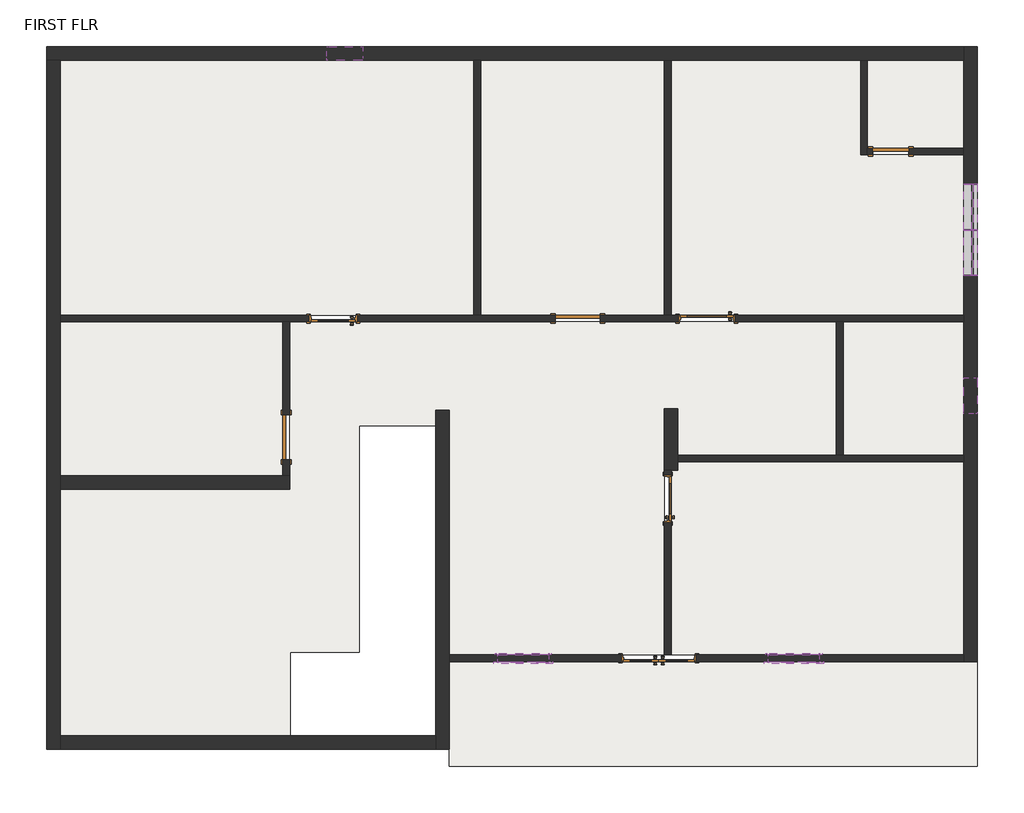
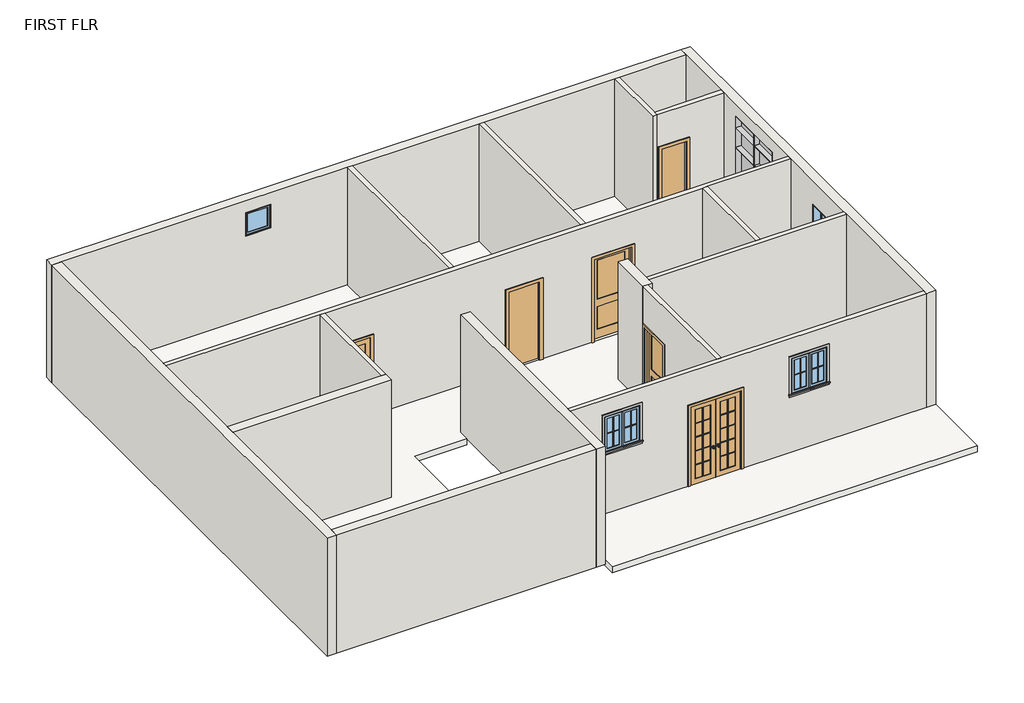
# One storey, incomplete: 22 members, 17 walls, 8 plates, 8 proxies, 7 doors, 4 windows, 2 slabs.
"""IFC4 building model written with IfcOpenShell, lengths in millimetres."""

from ifc_helpers import new_model, si_unit, frame, origin, place, context, project, spatial, polyline, outline, extrude, faceted_brep, transform, mapped, element, save
from components import muntin_pattern_2x2_muntin_pattern_2x2_b3fe6957, muntin_pattern_2x2_muntin_pattern_2x2_3e0ecaf2, trim_window_exterior_flat_with_sill_41619996, trim_window_interior_flat_picture_frame_51c85655, door_interior_double_full_glass_wood_double_door_glass_4_x_7_49a53587, door_d6fdea04, door_45c5d68b, door_049a69ed, door_d8f5dbb5, single_flush_bathroom_2_x_7_0bf9f8da, member_a87dc375, member_05d02c6e, member_049ff311, member_f4ca0770, member_d90fa784, member_091456ab, member_579a4f36, member_b53b5e8d, member_0fd823d9, member_acbd6ca0, system_panel_glazed_6813505b, system_panel_glazed_a35be92d, system_panel_glazed_bfd0fd53, system_panel_glazed_aaa2c267, window_80340324, window_a598f463

model = new_model("IFC4")

# Units and contexts
model_context = context("Model", 3, world=origin())
ifc_project = project(units=[si_unit("LENGTHUNIT", "METRE", prefix="MILLI")], contexts=[model_context])

# Site, building, storey
site = spatial("IfcSite", under=ifc_project)
building = spatial("IfcBuilding", under=site)
storey = spatial("IfcBuildingStorey", under=building, Name="FIRST FLR", Elevation=3352.8)

# Proxies
placement = place(None, origin())
muntin_pattern_2x2_muntin_pattern_2x2_shape = muntin_pattern_2x2_muntin_pattern_2x2_b3fe6957(model_context)
element("IfcBuildingElementProxy", 1, Name="Muntin Pattern_2x2 : Muntin Pattern_2x2", ObjectType="Muntin Pattern_2x2 : Muntin Pattern_2x2", at=placement, inside=storey, context=model_context, shape_type="MappedRepresentation", body=[
    mapped(muntin_pattern_2x2_muntin_pattern_2x2_shape, transform((2513.7983119, -4729.2803142, 5044.7639332), x_axis=(-1.0, 0.0, 0.0), y_axis=(0.0, -1.0, 0.0), z_axis=(0.0, 0.0, 1.0))),
])
element("IfcBuildingElementProxy", 2, Name="Muntin Pattern_2x2 : Muntin Pattern_2x2", ObjectType="Muntin Pattern_2x2 : Muntin Pattern_2x2", at=placement, inside=storey, context=model_context, shape_type="MappedRepresentation", body=[
    mapped(muntin_pattern_2x2_muntin_pattern_2x2_shape, transform((-2066.5321058, -4729.2803142, 5133.4876804), x_axis=(-1.0, 0.0, 0.0), y_axis=(0.0, -1.0, 0.0), z_axis=(0.0, 0.0, 1.0))),
])
muntin_pattern_2x2_muntin_pattern_2x2_2_shape = muntin_pattern_2x2_muntin_pattern_2x2_3e0ecaf2(model_context)
element("IfcBuildingElementProxy", 3, Name="Muntin Pattern_2x2 : Muntin Pattern_2x2", ObjectType="Muntin Pattern_2x2 : Muntin Pattern_2x2", at=placement, inside=storey, context=model_context, shape_type="MappedRepresentation", body=[
    mapped(muntin_pattern_2x2_muntin_pattern_2x2_2_shape, transform((2085.1733119, -4729.2803142, 5044.7639332), x_axis=(1.0, 0.0, 0.0), y_axis=(0.0, 1.0, 0.0), z_axis=(0.0, 0.0, 1.0))),
])
element("IfcBuildingElementProxy", 4, Name="Muntin Pattern_2x2 : Muntin Pattern_2x2", ObjectType="Muntin Pattern_2x2 : Muntin Pattern_2x2", at=placement, inside=storey, context=model_context, shape_type="MappedRepresentation", body=[
    mapped(muntin_pattern_2x2_muntin_pattern_2x2_2_shape, transform((-2495.1571058, -4729.2803142, 5133.4876804), x_axis=(1.0, 0.0, 0.0), y_axis=(0.0, 1.0, 0.0), z_axis=(0.0, 0.0, 1.0))),
])
trim_window_exterior_flat_with_sill_shape = trim_window_exterior_flat_with_sill_41619996(model_context)
element("IfcBuildingElementProxy", 5, Name="Trim-Window-Exterior-Flat : with Sill", ObjectType="Trim-Window-Exterior-Flat : with Sill", at=placement, inside=storey, context=model_context, shape_type="MappedRepresentation", body=[
    mapped(trim_window_exterior_flat_with_sill_shape, transform((2299.4858119, -4738.8053142, 5889.3139332), x_axis=(1.0, 0.0, 0.0), y_axis=(0.0, 0.0, 1.0), z_axis=(0.0, -1.0, 0.0))),
])
element("IfcBuildingElementProxy", 6, Name="Trim-Window-Exterior-Flat : with Sill", ObjectType="Trim-Window-Exterior-Flat : with Sill", at=placement, inside=storey, context=model_context, shape_type="MappedRepresentation", body=[
    mapped(trim_window_exterior_flat_with_sill_shape, transform((-2280.8446058, -4738.8053142, 5978.0376804), x_axis=(1.0, 0.0, 0.0), y_axis=(0.0, 0.0, 1.0), z_axis=(0.0, -1.0, 0.0))),
])
trim_window_interior_flat_picture_frame_shape = trim_window_interior_flat_picture_frame_51c85655(model_context)
element("IfcBuildingElementProxy", 7, Name="Trim-Window-Interior-Flat : Picture Frame", ObjectType="Trim-Window-Interior-Flat : Picture Frame", at=placement, inside=storey, context=model_context, shape_type="MappedRepresentation", body=[
    mapped(trim_window_interior_flat_picture_frame_shape, transform((2299.4858119, -4624.5053142, 5889.3139332), x_axis=(-1.0, 0.0, 0.0), y_axis=(0.0, 0.0, 1.0), z_axis=(0.0, 1.0, 0.0))),
])
element("IfcBuildingElementProxy", 8, Name="Trim-Window-Interior-Flat : Picture Frame", ObjectType="Trim-Window-Interior-Flat : Picture Frame", at=placement, inside=storey, context=model_context, shape_type="MappedRepresentation", body=[
    mapped(trim_window_interior_flat_picture_frame_shape, transform((-2280.8446058, -4624.5053142, 5978.0376804), x_axis=(-1.0, 0.0, 0.0), y_axis=(0.0, 0.0, 1.0), z_axis=(0.0, 1.0, 0.0))),
])

# Doors
door_interior_double_full_glass_wood_double_door_glass_4_x_7_shape = door_interior_double_full_glass_wood_double_door_glass_4_x_7_49a53587(model_context)
element("IfcDoor", 9, ObjectType="Door-Interior-Double-Full Glass-Wood : DOUBLE DOOR GLASS 4' X 7'", at=placement, inside=storey, context=model_context, shape_type="MappedRepresentation", body=[
    mapped(door_interior_double_full_glass_wood_double_door_glass_4_x_7_shape, transform((13.4858119, -4684.8303142, 3352.8), x_axis=(-1.0, 0.0, 0.0), y_axis=(0.0, -1.0, 0.0), z_axis=(0.0, 0.0, 1.0))),
])
door_shape = door_d6fdea04(model_context)
element("IfcDoor", 10, ObjectType="Door-Interior-Single-2_Panel-Wood : 30\" x 80\"", at=placement, inside=storey, context=model_context, shape_type="MappedRepresentation", body=[
    mapped(door_shape, transform((169.0608119, -1978.5424275, 3352.8), x_axis=(0.0, 1.0, 0.0), y_axis=(-1.0, 0.0, 0.0), z_axis=(0.0, 0.0, 1.0))),
])
door_2_shape = door_45c5d68b(model_context)
element("IfcDoor", 11, ObjectType="Door-Interior-Single-2_Panel-Wood : 30\" x 80\"", at=placement, inside=storey, context=model_context, shape_type="MappedRepresentation", body=[
    mapped(door_2_shape, transform((-5499.9044923, 1067.2421668, 3352.8), x_axis=(-1.0, 0.0, 0.0), y_axis=(0.0, -1.0, 0.0), z_axis=(0.0, 0.0, 1.0))),
])
door_3_shape = door_049a69ed(model_context)
element("IfcDoor", 12, ObjectType="Door-Interior-Single-2_Panel-Wood : 36\" x 84\"", at=placement, inside=storey, context=model_context, shape_type="MappedRepresentation", body=[
    mapped(door_3_shape, transform((824.7020146, 1073.5921668, 3352.8), x_axis=(-1.0, 0.0, 0.0), y_axis=(0.0, -1.0, 0.0), z_axis=(0.0, 0.0, 1.0))),
])
door_4_shape = door_d8f5dbb5(model_context)
element("IfcDoor", 13, ObjectType="Single-Flush : 30\" x 80\"", at=placement, inside=storey, context=model_context, shape_type="MappedRepresentation", body=[
    mapped(door_4_shape, transform((-1359.6979854, 1070.4171668, 3352.8), x_axis=(1.0, 0.0, 0.0), y_axis=(0.0, 1.0, 0.0), z_axis=(0.0, 0.0, 1.0))),
])
element("IfcDoor", 14, ObjectType="Single-Flush : 30\" x 80\"", at=placement, inside=storey, context=model_context, shape_type="MappedRepresentation", body=[
    mapped(door_4_shape, transform((-6295.715751, -942.6707851, 3352.8), x_axis=(0.0, 1.0, 0.0), y_axis=(-1.0, 0.0, 0.0), z_axis=(0.0, 0.0, 1.0))),
])
single_flush_bathroom_2_x_7_shape = single_flush_bathroom_2_x_7_0bf9f8da(model_context)
element("IfcDoor", 15, ObjectType="Single-Flush : BATHROOM 2' X 7'", at=placement, inside=storey, context=model_context, shape_type="MappedRepresentation", body=[
    mapped(single_flush_bathroom_2_x_7_shape, transform((3941.8301763, 3897.1946858, 3352.8), x_axis=(-1.0, 0.0, 0.0), y_axis=(0.0, -1.0, 0.0), z_axis=(0.0, 0.0, 1.0))),
])

# Members
member_shape = member_a87dc375(model_context)
element("IfcMember", 16, ObjectType="Rectangular Mullion : 2.5\" x 5\" rectangular", at=placement, inside=storey, context=model_context, shape_type="MappedRepresentation", body=[
    mapped(member_shape, transform((5293.034249, 2571.0346634, 3352.8), x_axis=(0.0, -1.0, 0.0), y_axis=(-1.0, 0.0, 0.0), z_axis=(0.0, 0.0, -1.0))),
])
member_2_shape = member_05d02c6e(model_context)
element("IfcMember", 17, ObjectType="Rectangular Mullion : 2.5\" x 5\" rectangular", at=placement, inside=storey, context=model_context, shape_type="MappedRepresentation", body=[
    mapped(member_2_shape, transform((5293.034249, 2571.0346634, 4216.4), x_axis=(0.0, -1.0, 0.0), y_axis=(-1.0, 0.0, 0.0), z_axis=(0.0, 0.0, -1.0))),
])
member_3_shape = member_049ff311(model_context)
element("IfcMember", 18, ObjectType="Rectangular Mullion : 2.5\" x 5\" rectangular", at=placement, inside=storey, context=model_context, shape_type="MappedRepresentation", body=[
    mapped(member_3_shape, transform((5293.034249, 1793.1596634, 3352.8), x_axis=(0.0, -1.0, 0.0), y_axis=(-1.0, 0.0, 0.0), z_axis=(0.0, 0.0, -1.0))),
])
member_4_shape = member_f4ca0770(model_context)
element("IfcMember", 19, ObjectType="Rectangular Mullion : 2.5\" x 5\" rectangular", at=placement, inside=storey, context=model_context, shape_type="MappedRepresentation", body=[
    mapped(member_4_shape, transform((5293.034249, 3348.9096634, 5283.2), x_axis=(0.0, 1.0, 0.0), y_axis=(-1.0, 0.0, 0.0), z_axis=(0.0, 0.0, 1.0))),
])
element("IfcMember", 20, ObjectType="Rectangular Mullion : 2.5\" x 5\" rectangular", at=placement, inside=storey, context=model_context, shape_type="MappedRepresentation", body=[
    mapped(member_4_shape, transform((5293.034249, 1793.1596634, 4216.4), x_axis=(0.0, -1.0, 0.0), y_axis=(-1.0, 0.0, 0.0), z_axis=(0.0, 0.0, -1.0))),
])
element("IfcMember", 21, ObjectType="Rectangular Mullion : 2.5\" x 5\" rectangular", at=placement, inside=storey, context=model_context, shape_type="MappedRepresentation", body=[
    mapped(member_3_shape, transform((5293.034249, 3348.9096634, 4216.4), x_axis=(0.0, 1.0, 0.0), y_axis=(-1.0, 0.0, 0.0), z_axis=(0.0, 0.0, 1.0))),
])
member_5_shape = member_d90fa784(model_context)
element("IfcMember", 22, ObjectType="Rectangular Mullion : 2.5\" x 5\" rectangular", at=placement, inside=storey, context=model_context, shape_type="MappedRepresentation", body=[
    mapped(member_5_shape, transform((5293.034249, 1800.3986634, 6096.0), x_axis=(0.0, 0.0, 1.0), y_axis=(-1.0, 0.0, 0.0), z_axis=(0.0, -1.0, 0.0))),
])
element("IfcMember", 23, ObjectType="Rectangular Mullion : 2.5\" x 5\" rectangular", at=placement, inside=storey, context=model_context, shape_type="MappedRepresentation", body=[
    mapped(member_5_shape, transform((5293.034249, 2574.6541634, 6096.0), x_axis=(0.0, 0.0, 1.0), y_axis=(-1.0, 0.0, 0.0), z_axis=(0.0, -1.0, 0.0))),
])
element("IfcMember", 24, ObjectType="Rectangular Mullion : 2.5\" x 5\" rectangular", at=placement, inside=storey, context=model_context, shape_type="MappedRepresentation", body=[
    mapped(member_5_shape, transform((5293.034249, 3341.6706634, 3352.8), x_axis=(0.0, 0.0, -1.0), y_axis=(-1.0, 0.0, 0.0), z_axis=(0.0, 1.0, 0.0))),
])
element("IfcMember", 25, ObjectType="Rectangular Mullion : 2.5\" x 5\" rectangular", at=placement, inside=storey, context=model_context, shape_type="MappedRepresentation", body=[
    mapped(member_5_shape, transform((5293.034249, 2567.4151634, 3352.8), x_axis=(0.0, 0.0, -1.0), y_axis=(-1.0, 0.0, 0.0), z_axis=(0.0, 1.0, 0.0))),
])
member_6_shape = member_091456ab(model_context)
element("IfcMember", 26, ObjectType="Rectangular Mullion : 2.5\" x 5\" rectangular", at=placement, inside=storey, context=model_context, shape_type="MappedRepresentation", body=[
    mapped(member_6_shape, transform((5293.034249, 2574.6541634, 5283.2), x_axis=(0.0, 0.0, 1.0), y_axis=(-1.0, 0.0, 0.0), z_axis=(0.0, -1.0, 0.0))),
])
element("IfcMember", 27, ObjectType="Rectangular Mullion : 2.5\" x 5\" rectangular", at=placement, inside=storey, context=model_context, shape_type="MappedRepresentation", body=[
    mapped(member_6_shape, transform((5293.034249, 1800.3986634, 5283.2), x_axis=(0.0, 0.0, 1.0), y_axis=(-1.0, 0.0, 0.0), z_axis=(0.0, -1.0, 0.0))),
])
element("IfcMember", 28, ObjectType="Rectangular Mullion : 2.5\" x 5\" rectangular", at=placement, inside=storey, context=model_context, shape_type="MappedRepresentation", body=[
    mapped(member_6_shape, transform((5293.034249, 2574.6541634, 4216.4), x_axis=(0.0, 0.0, 1.0), y_axis=(-1.0, 0.0, 0.0), z_axis=(0.0, -1.0, 0.0))),
])
element("IfcMember", 29, ObjectType="Rectangular Mullion : 2.5\" x 5\" rectangular", at=placement, inside=storey, context=model_context, shape_type="MappedRepresentation", body=[
    mapped(member_6_shape, transform((5293.034249, 1800.3986634, 4216.4), x_axis=(0.0, 0.0, 1.0), y_axis=(-1.0, 0.0, 0.0), z_axis=(0.0, -1.0, 0.0))),
])
element("IfcMember", 30, ObjectType="Rectangular Mullion : 2.5\" x 5\" rectangular", at=placement, inside=storey, context=model_context, shape_type="MappedRepresentation", body=[
    mapped(member_6_shape, transform((5293.034249, 2574.6541634, 5791.2), x_axis=(0.0, 0.0, 1.0), y_axis=(-1.0, 0.0, 0.0), z_axis=(0.0, -1.0, 0.0))),
])
element("IfcMember", 31, ObjectType="Rectangular Mullion : 2.5\" x 5\" rectangular", at=placement, inside=storey, context=model_context, shape_type="MappedRepresentation", body=[
    mapped(member_6_shape, transform((5293.034249, 1800.3986634, 5791.2), x_axis=(0.0, 0.0, 1.0), y_axis=(-1.0, 0.0, 0.0), z_axis=(0.0, -1.0, 0.0))),
])
member_7_shape = member_579a4f36(model_context)
element("IfcMember", 32, ObjectType="Rectangular Mullion : 2.5\" x 5\" rectangular", at=placement, inside=storey, context=model_context, shape_type="MappedRepresentation", body=[
    mapped(member_7_shape, transform((5293.034249, 1793.1596634, 5791.2), x_axis=(0.0, -1.0, 0.0), y_axis=(-1.0, 0.0, 0.0), z_axis=(0.0, 0.0, -1.0))),
])
element("IfcMember", 33, ObjectType="Rectangular Mullion : 2.5\" x 5\" rectangular", at=placement, inside=storey, context=model_context, shape_type="MappedRepresentation", body=[
    mapped(member_7_shape, transform((5293.034249, 3348.9096634, 6096.0), x_axis=(0.0, 1.0, 0.0), y_axis=(-1.0, 0.0, 0.0), z_axis=(0.0, 0.0, 1.0))),
])
member_8_shape = member_b53b5e8d(model_context)
element("IfcMember", 34, ObjectType="Rectangular Mullion : 2.5\" x 5\" rectangular", at=placement, inside=storey, context=model_context, shape_type="MappedRepresentation", body=[
    mapped(member_8_shape, transform((5293.034249, 2571.0346634, 5791.2), x_axis=(0.0, -1.0, 0.0), y_axis=(-1.0, 0.0, 0.0), z_axis=(0.0, 0.0, -1.0))),
])
member_9_shape = member_0fd823d9(model_context)
element("IfcMember", 35, ObjectType="Rectangular Mullion : 2.5\" x 5\" rectangular", at=placement, inside=storey, context=model_context, shape_type="MappedRepresentation", body=[
    mapped(member_9_shape, transform((5293.034249, 2571.0346634, 5283.2), x_axis=(0.0, -1.0, 0.0), y_axis=(-1.0, 0.0, 0.0), z_axis=(0.0, 0.0, -1.0))),
])
member_10_shape = member_acbd6ca0(model_context)
element("IfcMember", 36, ObjectType="Rectangular Mullion : 2.5\" x 5\" rectangular", at=placement, inside=storey, context=model_context, shape_type="MappedRepresentation", body=[
    mapped(member_10_shape, transform((5293.034249, 1793.1596634, 5283.2), x_axis=(0.0, -1.0, 0.0), y_axis=(-1.0, 0.0, 0.0), z_axis=(0.0, 0.0, -1.0))),
])
element("IfcMember", 37, ObjectType="Rectangular Mullion : 2.5\" x 5\" rectangular", at=placement, inside=storey, context=model_context, shape_type="MappedRepresentation", body=[
    mapped(member_10_shape, transform((5293.034249, 3348.9096634, 5791.2), x_axis=(0.0, 1.0, 0.0), y_axis=(-1.0, 0.0, 0.0), z_axis=(0.0, 0.0, 1.0))),
])

# Plates
system_panel_glazed_shape = system_panel_glazed_6813505b(model_context)
element("IfcPlate", 38, ObjectType="System Panel : Glazed", at=placement, inside=storey, context=model_context, shape_type="MappedRepresentation", body=[
    mapped(system_panel_glazed_shape, transform((5293.034249, 2958.1624134, 3360.039), x_axis=(0.0, -1.0, 0.0), y_axis=(1.0, 0.0, 0.0), z_axis=(0.0, 0.0, 1.0))),
])
element("IfcPlate", 39, ObjectType="System Panel : Glazed", at=placement, inside=storey, context=model_context, shape_type="MappedRepresentation", body=[
    mapped(system_panel_glazed_shape, transform((5293.034249, 2183.9069134, 3360.039), x_axis=(0.0, -1.0, 0.0), y_axis=(1.0, 0.0, 0.0), z_axis=(0.0, 0.0, 1.0))),
])
system_panel_glazed_2_shape = system_panel_glazed_a35be92d(model_context)
element("IfcPlate", 40, ObjectType="System Panel : Glazed", at=placement, inside=storey, context=model_context, shape_type="MappedRepresentation", body=[
    mapped(system_panel_glazed_2_shape, transform((5293.034249, 2958.1624134, 4220.0195), x_axis=(0.0, -1.0, 0.0), y_axis=(1.0, 0.0, 0.0), z_axis=(0.0, 0.0, 1.0))),
])
element("IfcPlate", 41, ObjectType="System Panel : Glazed", at=placement, inside=storey, context=model_context, shape_type="MappedRepresentation", body=[
    mapped(system_panel_glazed_2_shape, transform((5293.034249, 2183.9069134, 4220.0195), x_axis=(0.0, -1.0, 0.0), y_axis=(1.0, 0.0, 0.0), z_axis=(0.0, 0.0, 1.0))),
])
system_panel_glazed_3_shape = system_panel_glazed_bfd0fd53(model_context)
element("IfcPlate", 42, ObjectType="System Panel : Glazed", at=placement, inside=storey, context=model_context, shape_type="MappedRepresentation", body=[
    mapped(system_panel_glazed_3_shape, transform((5293.034249, 2958.1624134, 5286.8195), x_axis=(0.0, -1.0, 0.0), y_axis=(1.0, 0.0, 0.0), z_axis=(0.0, 0.0, 1.0))),
])
element("IfcPlate", 43, ObjectType="System Panel : Glazed", at=placement, inside=storey, context=model_context, shape_type="MappedRepresentation", body=[
    mapped(system_panel_glazed_3_shape, transform((5293.034249, 2183.9069134, 5286.8195), x_axis=(0.0, -1.0, 0.0), y_axis=(1.0, 0.0, 0.0), z_axis=(0.0, 0.0, 1.0))),
])
system_panel_glazed_4_shape = system_panel_glazed_aaa2c267(model_context)
element("IfcPlate", 44, ObjectType="System Panel : Glazed", at=placement, inside=storey, context=model_context, shape_type="MappedRepresentation", body=[
    mapped(system_panel_glazed_4_shape, transform((5293.034249, 2958.1624134, 5794.8195), x_axis=(0.0, -1.0, 0.0), y_axis=(1.0, 0.0, 0.0), z_axis=(0.0, 0.0, 1.0))),
])
element("IfcPlate", 45, ObjectType="System Panel : Glazed", at=placement, inside=storey, context=model_context, shape_type="MappedRepresentation", body=[
    mapped(system_panel_glazed_4_shape, transform((5293.034249, 2183.9069134, 5794.8195), x_axis=(0.0, -1.0, 0.0), y_axis=(1.0, 0.0, 0.0), z_axis=(0.0, 0.0, 1.0))),
])

# Slabs
element("IfcSlab", 46, ObjectType="MARBLE FLOORING 6\"", at=placement, inside=storey, context=model_context, shape_type="SweptSolid", body=[
    extrude(outline(polyline([(-3118.6544923, 5446.5946858), (-3118.6544923, 1127.5671668), (-10124.765751, 1127.5671668), (-10124.765751, 5446.5946858), (-3118.6544923, 5446.5946858)])), frame((0.0, 0.0, 3200.4), z_axis=(0.0, 0.0, 1.0), x_axis=(1.0, 0.0, 0.0)), (0.0, 0.0, 1.0), 152.4),
    extrude(outline(polyline([(107.1520146, 5446.5946858), (107.1520146, 1127.5671668), (-3004.3544923, 1127.5671668), (-3004.3544923, 5446.5946858), (107.1520146, 5446.5946858)])), frame((0.0, 0.0, 3200.4), z_axis=(0.0, 0.0, 1.0), x_axis=(1.0, 0.0, 0.0)), (0.0, 0.0, 1.0), 152.4),
    extrude(outline(polyline([(3427.4801763, 5446.5946858), (3427.4801763, 3840.0446858), (5178.734249, 3840.0446858), (5178.734249, 1127.5671668), (221.4520146, 1127.5671668), (221.4520146, 5446.5946858), (3427.4801763, 5446.5946858)])), frame((0.0, 0.0, 3200.4), z_axis=(0.0, 0.0, 1.0), x_axis=(1.0, 0.0, 0.0)), (0.0, 0.0, 1.0), 152.4),
    extrude(outline(polyline([(5178.734249, 5446.5946858), (5178.734249, 3954.3446858), (3541.7801763, 3954.3446858), (3541.7801763, 5446.5946858), (5178.734249, 5446.5946858)])), frame((0.0, 0.0, 3200.4), z_axis=(0.0, 0.0, 1.0), x_axis=(1.0, 0.0, 0.0)), (0.0, 0.0, 1.0), 152.4),
    extrude(outline(polyline([(5178.734249, 1013.2671668), (5178.734249, -1243.1716798), (3134.034249, -1243.1716798), (3134.034249, 1013.2671668), (5178.734249, 1013.2671668)])), frame((0.0, 0.0, 3200.4), z_axis=(0.0, 0.0, 1.0), x_axis=(1.0, 0.0, 0.0)), (0.0, 0.0, 1.0), 152.4),
    extrude(outline(polyline([(-6352.865751, 1013.2671668), (-6352.865751, -1590.3707851), (-10124.765751, -1590.3707851), (-10124.765751, 1013.2671668), (-6352.865751, 1013.2671668)])), frame((0.0, 0.0, 3200.4), z_axis=(0.0, 0.0, 1.0), x_axis=(1.0, 0.0, 0.0)), (0.0, 0.0, 1.0), 152.4),
    extrude(outline(polyline([(223.0358119, -4624.5053142), (223.0358119, -1495.9424275), (337.3358119, -1495.9424275), (337.3358119, -1357.4716798), (5178.734249, -1357.4716798), (5178.734249, -4624.5053142), (223.0358119, -4624.5053142)])), frame((0.0, 0.0, 3200.4), z_axis=(0.0, 0.0, 1.0), x_axis=(1.0, 0.0, 0.0)), (0.0, 0.0, 1.0), 152.4),
    extrude(outline(polyline([(-10124.765751, -1818.9707851), (-6238.565751, -1818.9707851), (-6238.565751, 1013.2671668), (3019.734249, 1013.2671668), (3019.734249, -1243.1716798), (337.3358119, -1243.1716798), (337.3358119, -454.5424275), (108.7358119, -454.5424275), (108.7358119, -4624.5053142), (-3538.1446058, -4624.5053142), (-3538.1446058, -484.3053142), (-3766.7446058, -484.3053142), (-3766.7446058, -746.7863315), (-5057.7237749, -746.7863315), (-5057.7237749, -4582.1863315), (-6226.1237749, -4582.1863315), (-6226.1237749, -5996.1053142), (-10124.765751, -5996.1053142), (-10124.765751, -1818.9707851)])), frame((0.0, 0.0, 3200.4), z_axis=(0.0, 0.0, 1.0), x_axis=(1.0, 0.0, 0.0)), (0.0, 0.0, 1.0), 152.4),
])
element("IfcSlab", 47, ObjectType="MARBLE FLOORING 6\"", at=placement, inside=storey, context=model_context, shape_type="SweptSolid", body=[
    extrude(outline(polyline([(5407.334249, -4738.8053142), (5407.334249, -6508.7205873), (-3538.1446058, -6508.7205873), (-3538.1446058, -4738.8053142), (5407.334249, -4738.8053142)])), frame((0.0, 0.0, 3302.0), z_axis=(0.0, 0.0, 1.0), x_axis=(1.0, 0.0, 0.0)), (0.0, 0.0, 1.0), 152.4),
])

# Walls
element("IfcWall", 48, at=placement, inside=storey, context=model_context, shape_type="SweptSolid", body=[
    extrude(outline(polyline([(-3766.7446058, -6224.7053142), (-10124.765751, -6224.7053142), (-10124.765751, -5996.1053142), (-3766.7446058, -5996.1053142), (-3766.7446058, -6224.7053142)])), frame((0.0, 0.0, 3352.8), z_axis=(0.0, 0.0, 1.0), x_axis=(1.0, 0.0, 0.0)), (0.0, 0.0, 1.0), 3048.0),
])
element("IfcWall", 49, at=placement, inside=storey, context=model_context, shape_type="Brep", body=[
    faceted_brep([(5407.334249, 5675.1946858, 6400.8), (5407.334249, -4738.8053142, 6400.8), (5407.334249, -4738.8053142, 3352.8), (5407.334249, 1793.1596634, 3352.8), (5407.334249, 1793.1596634, 6096.0), (5407.334249, 3348.9096634, 6096.0), (5407.334249, 3348.9096634, 3352.8), (5407.334249, 5675.1946858, 3352.8), (5407.334249, -538.3216798, 5791.2), (5407.334249, 71.2783202, 5791.2), (5407.334249, 71.2783202, 5181.6), (5407.334249, -538.3216798, 5181.6), (5178.734249, -4738.8053142, 6400.8), (5178.734249, -4624.5053142, 6400.8), (5178.734249, -1357.4716798, 6400.8), (5178.734249, -1243.1716798, 6400.8), (5178.734249, 1013.2671668, 6400.8), (5178.734249, 1127.5671668, 6400.8), (5178.734249, 3840.0446858, 6400.8), (5178.734249, 3954.3446858, 6400.8), (5178.734249, 5446.5946858, 6400.8), (5178.734249, 5675.1946858, 6400.8), (5178.734249, 5675.1946858, 3352.8), (5178.734249, 5446.5946858, 3352.8), (5178.734249, 3954.3446858, 3352.8), (5178.734249, 3840.0446858, 3352.8), (5178.734249, 3348.9096634, 3352.8), (5178.734249, 3348.9096634, 6096.0), (5178.734249, 1793.1596634, 6096.0), (5178.734249, 1793.1596634, 3352.8), (5178.734249, 1127.5671668, 3352.8), (5178.734249, 1013.2671668, 3352.8), (5178.734249, -1243.1716798, 3352.8), (5178.734249, -1357.4716798, 3352.8), (5178.734249, -4624.5053142, 3352.8), (5178.734249, -4738.8053142, 3352.8), (5178.734249, -538.3216798, 5791.2), (5178.734249, -538.3216798, 5181.6), (5178.734249, 71.2783202, 5181.6), (5178.734249, 71.2783202, 5791.2)], [[[0, 1, 2, 3, 4, 5, 6, 7], [8, 9, 10, 11]], [[12, 13, 14, 15, 16, 17, 18, 19, 20, 21, 22, 23, 24, 25, 26, 27, 28, 29, 30, 31, 32, 33, 34, 35], [36, 37, 38, 39]], [[2, 35, 34, 33, 32, 31, 30, 29, 3]], [[22, 7, 6, 26, 25, 24, 23]], [[1, 0, 21, 20, 19, 18, 17, 16, 15, 14, 13, 12]], [[2, 1, 12, 35]], [[0, 7, 22, 21]], [[5, 27, 26, 6]], [[27, 5, 4, 28]], [[28, 4, 3, 29]], [[37, 36, 8, 11]], [[38, 37, 11, 10]], [[39, 38, 10, 9]], [[36, 39, 9, 8]]]),
])
element("IfcWall", 50, at=placement, inside=storey, context=model_context, shape_type="Brep", body=[
    faceted_brep([(5178.734249, 5675.1946858, 3352.8), (-10353.365751, 5675.1946858, 3352.8), (-10353.365751, 5675.1946858, 6400.8), (5178.734249, 5675.1946858, 6400.8), (-5608.7434923, 5675.1946858, 6096.0), (-5608.7434923, 5675.1946858, 5486.4), (-4999.1434923, 5675.1946858, 5486.4), (-4999.1434923, 5675.1946858, 6096.0), (5178.734249, 5446.5946858, 3352.8), (5178.734249, 5446.5946858, 6400.8), (3541.7801763, 5446.5946858, 6400.8), (3427.4801763, 5446.5946858, 6400.8), (221.4520146, 5446.5946858, 6400.8), (107.1520146, 5446.5946858, 6400.8), (-3004.3544923, 5446.5946858, 6400.8), (-3118.6544923, 5446.5946858, 6400.8), (-10124.765751, 5446.5946858, 6400.8), (-10353.365751, 5446.5946858, 6400.8), (-10353.365751, 5446.5946858, 3352.8), (-10124.765751, 5446.5946858, 3352.8), (-3118.6544923, 5446.5946858, 3352.8), (-3004.3544923, 5446.5946858, 3352.8), (107.1520146, 5446.5946858, 3352.8), (221.4520146, 5446.5946858, 3352.8), (3427.4801763, 5446.5946858, 3352.8), (3541.7801763, 5446.5946858, 3352.8), (-5608.7434923, 5446.5946858, 6096.0), (-4999.1434923, 5446.5946858, 6096.0), (-4999.1434923, 5446.5946858, 5486.4), (-5608.7434923, 5446.5946858, 5486.4)], [[[0, 1, 2, 3], [4, 5, 6, 7]], [[8, 9, 10, 11, 12, 13, 14, 15, 16, 17, 18, 19, 20, 21, 22, 23, 24, 25], [26, 27, 28, 29]], [[1, 0, 8, 25, 24, 23, 22, 21, 20, 19, 18]], [[3, 2, 17, 16, 15, 14, 13, 12, 11, 10, 9]], [[0, 3, 9, 8]], [[2, 1, 18, 17]], [[5, 4, 26, 29]], [[6, 5, 29, 28]], [[7, 6, 28, 27]], [[4, 7, 27, 26]]]),
])
element("IfcWall", 51, at=placement, inside=storey, context=model_context, shape_type="Brep", body=[
    faceted_brep([(-10353.365751, 5446.5946858, 3352.8), (-10353.365751, -6224.7053142, 3352.8), (-10353.365751, -6224.7053142, 6400.8), (-10353.365751, 5446.5946858, 6400.8), (-10124.765751, 5446.5946858, 3352.8), (-10124.765751, 5446.5946858, 6400.8), (-10124.765751, 1127.5671668, 6400.8), (-10124.765751, 1013.2671668, 6400.8), (-10124.765751, -1590.3707851, 6400.8), (-10124.765751, -1818.9707851, 6400.8), (-10124.765751, -5996.1053142, 6400.8), (-10124.765751, -6224.7053142, 6400.8), (-10124.765751, -6224.7053142, 3352.8), (-10124.765751, -5996.1053142, 3352.8), (-10124.765751, -1818.9707851, 3352.8), (-10124.765751, -1590.3707851, 3352.8), (-10124.765751, 1013.2671668, 3352.8), (-10124.765751, 1127.5671668, 3352.8)], [[[0, 1, 2, 3]], [[4, 5, 6, 7, 8, 9, 10, 11, 12, 13, 14, 15, 16, 17]], [[1, 0, 4, 17, 16, 15, 14, 13, 12]], [[3, 2, 11, 10, 9, 8, 7, 6, 5]], [[0, 3, 5, 4]], [[2, 1, 12, 11]]]),
])
element("IfcWall", 52, at=placement, inside=storey, context=model_context, shape_type="Brep", body=[
    faceted_brep([(-10124.765751, -1818.9707851, 3352.8), (-6238.565751, -1818.9707851, 3352.8), (-6238.565751, -1818.9707851, 6400.8), (-10124.765751, -1818.9707851, 6400.8), (-10124.765751, -1590.3707851, 3352.8), (-10124.765751, -1590.3707851, 6400.8), (-6352.865751, -1590.3707851, 6400.8), (-6238.565751, -1590.3707851, 6400.8), (-6238.565751, -1590.3707851, 3352.8), (-6352.865751, -1590.3707851, 3352.8)], [[[0, 1, 2, 3]], [[4, 5, 6, 7, 8, 9]], [[1, 0, 4, 9, 8]], [[3, 2, 7, 6, 5]], [[0, 3, 5, 4]], [[2, 1, 8, 7]]]),
])
element("IfcWall", 53, at=placement, inside=storey, context=model_context, shape_type="Brep", body=[
    faceted_brep([(-3538.1446058, -6224.7053142, 3352.8), (-3538.1446058, -4738.8053142, 3352.8), (-3538.1446058, -4624.5053142, 3352.8), (-3538.1446058, -484.3053142, 3352.8), (-3538.1446058, -484.3053142, 6400.8), (-3538.1446058, -4624.5053142, 6400.8), (-3538.1446058, -4738.8053142, 6400.8), (-3538.1446058, -6224.7053142, 6400.8), (-3766.7446058, -6224.7053142, 3352.8), (-3766.7446058, -6224.7053142, 6400.8), (-3766.7446058, -5996.1053142, 6400.8), (-3766.7446058, -484.3053142, 6400.8), (-3766.7446058, -484.3053142, 3352.8), (-3766.7446058, -5996.1053142, 3352.8)], [[[0, 1, 2, 3, 4, 5, 6, 7]], [[8, 9, 10, 11, 12, 13]], [[3, 2, 1, 0, 8, 13, 12]], [[4, 3, 12, 11]], [[7, 6, 5, 4, 11, 10, 9]], [[0, 7, 9, 8]]]),
])
element("IfcWall", 54, at=placement, inside=storey, context=model_context, shape_type="Brep", body=[
    faceted_brep([(108.7358119, -454.5424275, 3352.8), (108.7358119, -1495.9424275, 3352.8), (108.7358119, -1495.9424275, 6400.8), (108.7358119, -454.5424275, 6400.8), (337.3358119, -454.5424275, 3352.8), (337.3358119, -454.5424275, 6400.8), (337.3358119, -1243.1716798, 6400.8), (337.3358119, -1357.4716798, 6400.8), (337.3358119, -1495.9424275, 6400.8), (337.3358119, -1495.9424275, 3352.8), (337.3358119, -1357.4716798, 3352.8), (337.3358119, -1243.1716798, 3352.8), (223.0358119, -1495.9424275, 3352.8), (223.0358119, -1495.9424275, 6400.8)], [[[0, 1, 2, 3]], [[4, 5, 6, 7, 8, 9, 10, 11]], [[1, 0, 4, 11, 10, 9, 12]], [[2, 1, 12, 9, 8, 13]], [[3, 2, 13, 8, 7, 6, 5]], [[0, 3, 5, 4]]]),
])
element("IfcWall", 55, ObjectType="INTERIOR WALL THICKNESS 4.5\"", at=placement, inside=storey, context=model_context, shape_type="Brep", body=[
    faceted_brep([(5178.734249, -1243.1716798, 3352.8), (3134.034249, -1243.1716798, 3352.8), (3019.734249, -1243.1716798, 3352.8), (337.3358119, -1243.1716798, 3352.8), (337.3358119, -1243.1716798, 6400.8), (3019.734249, -1243.1716798, 6400.8), (3134.034249, -1243.1716798, 6400.8), (5178.734249, -1243.1716798, 6400.8), (5178.734249, -1357.4716798, 3352.8), (5178.734249, -1357.4716798, 6400.8), (337.3358119, -1357.4716798, 6400.8), (337.3358119, -1357.4716798, 3352.8)], [[[0, 1, 2, 3, 4, 5, 6, 7]], [[8, 9, 10, 11]], [[3, 2, 1, 0, 8, 11]], [[7, 6, 5, 4, 10, 9]], [[0, 7, 9, 8]], [[4, 3, 11, 10]]]),
])
element("IfcWall", 56, ObjectType="INTERIOR WALL THICKNESS 4.5\"", at=placement, inside=storey, context=model_context, shape_type="SweptSolid", body=[
    extrude(outline(polyline([(3019.734249, -1243.1716798), (3019.734249, 1013.2671668), (3134.034249, 1013.2671668), (3134.034249, -1243.1716798), (3019.734249, -1243.1716798)])), frame((0.0, 0.0, 3352.8), z_axis=(0.0, 0.0, 1.0), x_axis=(1.0, 0.0, 0.0)), (0.0, 0.0, 1.0), 3048.0),
])
element("IfcWall", 57, ObjectType="INTERIOR WALL THICKNESS 4.5\"", at=placement, inside=storey, context=model_context, shape_type="Brep", body=[
    faceted_brep([(3427.4801763, 5446.5946858, 3352.8), (3427.4801763, 3840.0446858, 3352.8), (3427.4801763, 3840.0446858, 6400.8), (3427.4801763, 5446.5946858, 6400.8), (3541.7801763, 5446.5946858, 3352.8), (3541.7801763, 5446.5946858, 6400.8), (3541.7801763, 3954.3446858, 6400.8), (3541.7801763, 3840.0446858, 6400.8), (3541.7801763, 3840.0446858, 3352.8), (3541.7801763, 3954.3446858, 3352.8)], [[[0, 1, 2, 3]], [[4, 5, 6, 7, 8, 9]], [[1, 0, 4, 9, 8]], [[3, 2, 7, 6, 5]], [[0, 3, 5, 4]], [[2, 1, 8, 7]]]),
])
element("IfcWall", 58, ObjectType="INTERIOR WALL THICKNESS 4.5\"", at=placement, inside=storey, context=model_context, shape_type="SweptSolid", body=[
    extrude(outline(polyline([(3352.8, 3541.7801763), (3352.8, 3637.0301763), (5486.4, 3637.0301763), (5486.4, 4246.6301763), (3352.8, 4246.6301763), (3352.8, 5178.734249), (6400.8, 5178.734249), (6400.8, 3541.7801763), (3352.8, 3541.7801763)])), frame((0.0, 3840.0446858, 0.0), z_axis=(0.0, 1.0, 0.0), x_axis=(0.0, 0.0, 1.0)), (0.0, 0.0, 1.0), 114.3),
])
element("IfcWall", 59, ObjectType="INTERIOR WALL THICKNESS 4.5\"", at=placement, inside=storey, context=model_context, shape_type="Brep", body=[
    faceted_brep([(5178.734249, 1013.2671668, 6400.8), (3134.034249, 1013.2671668, 6400.8), (3019.734249, 1013.2671668, 6400.8), (-6238.565751, 1013.2671668, 6400.8), (-6352.865751, 1013.2671668, 6400.8), (-10124.765751, 1013.2671668, 6400.8), (-10124.765751, 1013.2671668, 3352.8), (-6352.865751, 1013.2671668, 3352.8), (-6238.565751, 1013.2671668, 3352.8), (-5906.3044923, 1013.2671668, 3352.8), (-5906.3044923, 1013.2671668, 5410.2), (-5093.5044923, 1013.2671668, 5410.2), (-5093.5044923, 1013.2671668, 3352.8), (-1740.6979854, 1013.2671668, 3352.8), (-1740.6979854, 1013.2671668, 5384.8), (-978.6979854, 1013.2671668, 5384.8), (-978.6979854, 1013.2671668, 3352.8), (342.1020146, 1013.2671668, 3352.8), (342.1020146, 1013.2671668, 5511.8), (1307.3020146, 1013.2671668, 5511.8), (1307.3020146, 1013.2671668, 3352.8), (3019.734249, 1013.2671668, 3352.8), (3134.034249, 1013.2671668, 3352.8), (5178.734249, 1013.2671668, 3352.8), (-10124.765751, 1127.5671668, 6400.8), (-3118.6544923, 1127.5671668, 6400.8), (-3004.3544923, 1127.5671668, 6400.8), (107.1520146, 1127.5671668, 6400.8), (221.4520146, 1127.5671668, 6400.8), (5178.734249, 1127.5671668, 6400.8), (5178.734249, 1127.5671668, 3352.8), (1307.3020146, 1127.5671668, 3352.8), (1307.3020146, 1127.5671668, 5511.8), (342.1020146, 1127.5671668, 5511.8), (342.1020146, 1127.5671668, 3352.8), (221.4520146, 1127.5671668, 3352.8), (107.1520146, 1127.5671668, 3352.8), (-978.6979854, 1127.5671668, 3352.8), (-978.6979854, 1127.5671668, 5384.8), (-1740.6979854, 1127.5671668, 5384.8), (-1740.6979854, 1127.5671668, 3352.8), (-3004.3544923, 1127.5671668, 3352.8), (-3118.6544923, 1127.5671668, 3352.8), (-5093.5044923, 1127.5671668, 3352.8), (-5093.5044923, 1127.5671668, 5410.2), (-5906.3044923, 1127.5671668, 5410.2), (-5906.3044923, 1127.5671668, 3352.8), (-10124.765751, 1127.5671668, 3352.8)], [[[0, 1, 2, 3, 4, 5, 6, 7, 8, 9, 10, 11, 12, 13, 14, 15, 16, 17, 18, 19, 20, 21, 22, 23]], [[24, 25, 26, 27, 28, 29, 30, 31, 32, 33, 34, 35, 36, 37, 38, 39, 40, 41, 42, 43, 44, 45, 46, 47]], [[6, 47, 46, 9, 8, 7]], [[30, 23, 22, 21, 20, 31]], [[12, 43, 42, 41, 40, 13]], [[16, 37, 36, 35, 34, 17]], [[5, 4, 3, 2, 1, 0, 29, 28, 27, 26, 25, 24]], [[0, 23, 30, 29]], [[6, 5, 24, 47]], [[45, 10, 9, 46]], [[10, 45, 44, 11]], [[11, 44, 43, 12]], [[38, 37, 16, 15]], [[39, 38, 15, 14]], [[40, 39, 14, 13]], [[33, 18, 17, 34]], [[18, 33, 32, 19]], [[19, 32, 31, 20]]]),
])
element("IfcWall", 60, ObjectType="INTERIOR WALL THICKNESS 4.5\"", at=placement, inside=storey, context=model_context, shape_type="SweptSolid", body=[
    extrude(outline(polyline([(107.1520146, 1127.5671668), (107.1520146, 5446.5946858), (221.4520146, 5446.5946858), (221.4520146, 1127.5671668), (107.1520146, 1127.5671668)])), frame((0.0, 0.0, 3352.8), z_axis=(0.0, 0.0, 1.0), x_axis=(1.0, 0.0, 0.0)), (0.0, 0.0, 1.0), 3048.0),
])
element("IfcWall", 61, ObjectType="INTERIOR WALL THICKNESS 4.5\"", at=placement, inside=storey, context=model_context, shape_type="SweptSolid", body=[
    extrude(outline(polyline([(-3118.6544923, 1127.5671668), (-3118.6544923, 5446.5946858), (-3004.3544923, 5446.5946858), (-3004.3544923, 1127.5671668), (-3118.6544923, 1127.5671668)])), frame((0.0, 0.0, 3352.8), z_axis=(0.0, 0.0, 1.0), x_axis=(1.0, 0.0, 0.0)), (0.0, 0.0, 1.0), 3048.0),
])
element("IfcWall", 62, ObjectType="INTERIOR WALL THICKNESS 4.5\"", at=placement, inside=storey, context=model_context, shape_type="SweptSolid", body=[
    extrude(outline(polyline([(1013.2671668, 3352.8), (-561.6707851, 3352.8), (-561.6707851, 5384.8), (-1323.6707851, 5384.8), (-1323.6707851, 3352.8), (-1590.3707851, 3352.8), (-1590.3707851, 6400.8), (1013.2671668, 6400.8), (1013.2671668, 3352.8)])), frame((-6352.865751, 0.0, 0.0), z_axis=(1.0, 0.0, 0.0), x_axis=(0.0, 1.0, 0.0)), (0.0, 0.0, 1.0), 114.3),
])
element("IfcWall", 63, ObjectType="INTERIOR WALL THICKNESS 4.5\"", at=placement, inside=storey, context=model_context, shape_type="Brep", body=[
    faceted_brep([(5178.734249, -4738.8053142, 6400.8), (-3538.1446058, -4738.8053142, 6400.8), (-3538.1446058, -4738.8053142, 3352.8), (-621.5141881, -4738.8053142, 3352.8), (-621.5141881, -4738.8053142, 5511.8), (648.4858119, -4738.8053142, 5511.8), (648.4858119, -4738.8053142, 3352.8), (5178.734249, -4738.8053142, 3352.8), (1867.6858119, -4738.8053142, 5889.3139332), (2731.2858119, -4738.8053142, 5889.3139332), (2731.2858119, -4738.8053142, 4974.9139332), (1867.6858119, -4738.8053142, 4974.9139332), (-2712.6446058, -4738.8053142, 5978.0376804), (-1849.0446058, -4738.8053142, 5978.0376804), (-1849.0446058, -4738.8053142, 5063.6376804), (-2712.6446058, -4738.8053142, 5063.6376804), (-3538.1446058, -4624.5053142, 6400.8), (108.7358119, -4624.5053142, 6400.8), (223.0358119, -4624.5053142, 6400.8), (5178.734249, -4624.5053142, 6400.8), (5178.734249, -4624.5053142, 3352.8), (648.4858119, -4624.5053142, 3352.8), (648.4858119, -4624.5053142, 5511.8), (-621.5141881, -4624.5053142, 5511.8), (-621.5141881, -4624.5053142, 3352.8), (-3538.1446058, -4624.5053142, 3352.8), (1867.6858119, -4624.5053142, 5889.3139332), (1867.6858119, -4624.5053142, 4974.9139332), (2731.2858119, -4624.5053142, 4974.9139332), (2731.2858119, -4624.5053142, 5889.3139332), (-2712.6446058, -4624.5053142, 5978.0376804), (-2712.6446058, -4624.5053142, 5063.6376804), (-1849.0446058, -4624.5053142, 5063.6376804), (-1849.0446058, -4624.5053142, 5978.0376804)], [[[0, 1, 2, 3, 4, 5, 6, 7], [8, 9, 10, 11], [12, 13, 14, 15]], [[16, 17, 18, 19, 20, 21, 22, 23, 24, 25], [26, 27, 28, 29], [30, 31, 32, 33]], [[2, 25, 24, 3]], [[20, 7, 6, 21]], [[1, 0, 19, 18, 17, 16]], [[0, 7, 20, 19]], [[2, 1, 16, 25]], [[23, 4, 3, 24]], [[4, 23, 22, 5]], [[5, 22, 21, 6]], [[27, 26, 8, 11]], [[28, 27, 11, 10]], [[29, 28, 10, 9]], [[26, 29, 9, 8]], [[31, 30, 12, 15]], [[32, 31, 15, 14]], [[33, 32, 14, 13]], [[30, 33, 13, 12]]]),
])
element("IfcWall", 64, ObjectType="INTERIOR WALL THICKNESS 4.5\"", at=placement, inside=storey, context=model_context, shape_type="SweptSolid", body=[
    extrude(outline(polyline([(-1495.9424275, 6400.8), (-1495.9424275, 3352.8), (-1572.1424275, 3352.8), (-1572.1424275, 5410.2), (-2384.9424275, 5410.2), (-2384.9424275, 3352.8), (-4624.5053142, 3352.8), (-4624.5053142, 6400.8), (-1495.9424275, 6400.8)])), frame((108.7358119, 0.0, 0.0), z_axis=(1.0, 0.0, 0.0), x_axis=(0.0, 1.0, 0.0)), (0.0, 0.0, 1.0), 114.3),
])

# Windows
window_shape = window_80340324(model_context)
element("IfcWindow", 65, ObjectType="Fixed : 24\" x 24\"", at=placement, inside=storey, context=model_context, shape_type="MappedRepresentation", body=[
    mapped(window_shape, transform((-5342.0434923, 5560.8946858, 4572.0), x_axis=(-1.0, 0.0, 0.0), y_axis=(0.0, -1.0, 0.0), z_axis=(0.0, 0.0, 1.0))),
])
element("IfcWindow", 66, ObjectType="Fixed : 24\" x 24\"", at=placement, inside=storey, context=model_context, shape_type="MappedRepresentation", body=[
    mapped(window_shape, transform((5293.034249, -271.6216798, 4267.2), x_axis=(0.0, -1.0, 0.0), y_axis=(1.0, 0.0, 0.0), z_axis=(0.0, 0.0, 1.0))),
])
window_2_shape = window_a598f463(model_context)
element("IfcWindow", 67, ObjectType="Window-Casement-Double : 34\" x 36\"", at=placement, inside=storey, context=model_context, shape_type="MappedRepresentation", body=[
    mapped(window_2_shape, transform((2299.4858119, -4681.6553142, 4060.5139332), x_axis=(-1.0, 0.0, 0.0), y_axis=(0.0, -1.0, 0.0), z_axis=(0.0, 0.0, 1.0))),
])
element("IfcWindow", 68, ObjectType="Window-Casement-Double : 34\" x 36\"", at=placement, inside=storey, context=model_context, shape_type="MappedRepresentation", body=[
    mapped(window_2_shape, transform((-2280.8446058, -4681.6553142, 4149.2376804), x_axis=(-1.0, 0.0, 0.0), y_axis=(0.0, -1.0, 0.0), z_axis=(0.0, 0.0, 1.0))),
])

save(model, "model.ifc")

# Revit data of these elements
# Type "Muntin Pattern_2x2 : Muntin Pattern_2x2"
#   Width [instance default] = 4' - 0"
#   Thickness = 0' - 0 1/2"
#   Height [instance default] = 4' - 0"
#   Distance = 0' - 0 3/4"
#   Interior Material [instance default] = none
#   Exterior Material [instance default] = none
#   Default Elevation = 0
# Type "Trim-Window-Exterior-Flat : with Sill"
#   Trim Width = 0' - 2 1/4"
#   Trim Thickness_Picture Frame = 0' - 1 1/4"
#   Trim Thickness_with Sill = 0' - 0 3/4"
#   Sill Thickness = 0' - 1 1/4"
#   Opening Width [instance default] = 2' - 0"
#   Opening Height [instance default] = 3' - 0"
#   Default Elevation = 4' - 0"
#   Sill = yes
#   Picture Frame = no
#   Trim Material [instance default] = none
# Type "Trim-Window-Interior-Flat : Picture Frame"
#   Trim Thickness_Picture Frame = 0' - 1 1/4"
#   Trim Width = 0' - 2 1/4"
#   Trim Thickness_with Sill = 0' - 0 3/4"
#   Sill Thickness = 0' - 1 1/4"
#   Opening Width [instance default] = 2' - 0"
#   Opening Height [instance default] = 3' - 0"
#   Default Elevation = 4' - 0"
#   Sill = no
#   Picture Frame = yes
#   Trim Material [instance default] = none
# Type "Door-Interior-Double-Full Glass-Wood : DOUBLE DOOR GLASS 4' X 7'"
#   Type Mark = "12"
#   Assembly Code = "C1020300"
#   Analytic Construction = "French door, wood frame with single glass"
#   Top Rail = 0' - 4 11/16"
#   Thickness = 0' - 1 3/8"
#   Thermal Resistance (R) = 1.0696 (h·ft²·°F)/BTU
#   Swing Angle [instance default] = 90.00°
#   Stiles = 0' - 4 3/4"
#   Rough Width = 4' - 2"
#   Rough Height = 7' - 1"
#   Panel Width = 2' - 0"
#   Height = 7' - 0"
#   Width = 4' - 0"
#   Heat Transfer Coefficient (U) = 0.9350 BTU/(h·ft²·°F)
#   Bottom Rail = 0' - 9 1/8"
#   Show Grill [instance default] = yes
#   Trim Material = Cherry
#   Panel Material = Cherry
#   Frame Material = Cherry
#   Door Handle Material = Aluminum
#   Visual Light Transmittance = 0
#   Solar Heat Gain Coefficient = 0
#   Wall Closure = (empty or 0)
#   Function = (empty or 0)
# Type "Door-Interior-Single-2_Panel-Wood : 30\" x 80\""
#   Type Mark = "14"
#   Assembly Code = "C1020300"
#   Analytic Construction = "Wooden"
#   Top Rail = 0' - 4 11/16"
#   Thickness = 0' - 1 3/8"
#   Thermal Resistance (R) = 2.5876 (h·ft²·°F)/BTU
#   Swing Angle [instance default] = 90.00°
#   Stiles = 0' - 4 3/4"
#   Rough Width = 2' - 8"
#   Rough Height = 6' - 9"
#   Lock Rail = 0' - 7 1/2"
#   Height = 6' - 8"
#   Width = 2' - 6"
#   Heat Transfer Coefficient (U) = 0.3865 BTU/(h·ft²·°F)
#   Bottom Rail = 0' - 9 1/8"
#   Trim Material = Cherry
#   Panel Material = Cherry
#   Frame Material = Cherry
#   Door Handle Material = Aluminum
#   Visual Light Transmittance = 0
#   Solar Heat Gain Coefficient = 0
#   Wall Closure = (empty or 0)
#   Function = (empty or 0)
# Type "Door-Interior-Single-2_Panel-Wood : 36\" x 84\""
#   Type Mark = "9"
#   Assembly Code = "C1020300"
#   Analytic Construction = "Wooden"
#   Top Rail = 0' - 4 11/16"
#   Thickness = 0' - 1 3/8"
#   Thermal Resistance (R) = 2.5876 (h·ft²·°F)/BTU
#   Swing Angle [instance default] = 90.00°
#   Stiles = 0' - 4 3/4"
#   Rough Width = 3' - 2"
#   Rough Height = 7' - 1"
#   Lock Rail = 0' - 7 1/2"
#   Height = 7' - 0"
#   Width = 3' - 0"
#   Heat Transfer Coefficient (U) = 0.3865 BTU/(h·ft²·°F)
#   Bottom Rail = 0' - 9 1/8"
#   Trim Material = Cherry
#   Panel Material = Cherry
#   Frame Material = Cherry
#   Door Handle Material = Aluminum
#   Visual Light Transmittance = 0
#   Solar Heat Gain Coefficient = 0
#   Wall Closure = (empty or 0)
#   Function = (empty or 0)
# Type "Single-Flush : 30\" x 80\""
#   Type Mark = "5"
#   Construction Type Id = "MDOOR"
#   Assembly Code = "C1020"
#   Analytic Construction = "Metal"
#   Thickness = 0' - 2"
#   Heat Transfer Coefficient (U) = 0.651978 BTU/(h·ft²·°F)
#   Height = 6' - 8"
#   Trim Projection Ext = 0' - 1"
#   Trim Projection Int = 0' - 1"
#   Trim Width = 0' - 3"
#   Width = 2' - 6"
#   Define Thermal Properties by = 1
#   Define Thermal Properties by = 1
#   Door Material = Door - Panel
#   Frame Material = Door - Frame
#   Visual Light Transmittance = 0
#   Solar Heat Gain Coefficient = 0
#   Function = (empty or 0)
#   Wall Closure = (empty or 0)
# Type "Single-Flush : BATHROOM 2' X 7'"
#   Type Mark = "8"
#   Construction Type Id = "MDOOR"
#   Assembly Code = "C1020"
#   Analytic Construction = "Metal"
#   Thickness = 0' - 2"
#   Heat Transfer Coefficient (U) = 0.651978 BTU/(h·ft²·°F)
#   Height = 7' - 0"
#   Trim Projection Ext = 0' - 1"
#   Trim Projection Int = 0' - 1"
#   Trim Width = 0' - 3"
#   Width = 2' - 0"
#   Define Thermal Properties by = 1
#   Door Material = Door - Panel
#   Frame Material = Door - Frame
#   Visual Light Transmittance = 0
#   Solar Heat Gain Coefficient = 0
#   Function = (empty or 0)
#   Wall Closure = (empty or 0)
# Type "Rectangular Mullion : 2.5\" x 5\" rectangular"
#   built-in parameter 1007304 = 0.75 (stored number, unit not read)
#   built-in parameter 1007301 = 0.011875 (stored number, unit not read)
#   built-in parameter 1007300 = 0.011875 (stored number, unit not read)
# Type "System Panel : Glazed"
#   Construction Type Id = "GSP4R"
#   Analytic Construction = "1/8 in Pilkington single glazing"
#   Visual Light Transmittance = 0.9
#   Solar Heat Gain Coefficient = 0.86
#   Heat Transfer Coefficient (U) = 1.18115 BTU/(h·ft²·°F)
#   Define Thermal Properties by = 1
# Type "MARBLE FLOORING 6\""
#   Assembly Code = "B1010"
#   Function = 0
#   Layers, outside or top first: 0' - 6" "MARBLE FLOORING 1'" (function 1)
# Type
#   Assembly Code = "B2010"
#   Layers, outside or top first: 0' - 9" "BEIGE COLOUR" (function 1)
# Type "INTERIOR WALL THICKNESS 4.5\""
#   Assembly Code = "B2010"
#   Layers, outside or top first: 0' - 4 1/2" "BEIGE COLOUR" (function 1)
# Type "Fixed : 24\" x 24\""
#   Type Mark = "3"
#   Construction Type Id = "GSP4R"
#   Assembly Code = "B2020100"
#   Analytic Construction = "1/8 in Pilkington single glazing"
#   Visual Light Transmittance = 0.9
#   Solar Heat Gain Coefficient = 0.78
#   Heat Transfer Coefficient (U) = 0.6496 BTU/(h·ft²·°F)
#   Height = 2' - 0"
#   Default Sill Height = 3' - 0"
#   Width = 2' - 0"
#   Window Inset = 0' - 0 3/4"
#   Define Thermal Properties by = 1
#   Define Thermal Properties by = 1
#   Glass Pane Material = Glass
#   Sash Material = Sash
#   Wall Closure = (empty or 0)
# Type "Window-Casement-Double : 34\" x 36\""
#   Type Mark = "14"
#   Fire Rating = "0.5h"
#   Assembly Code = "B2020100"
#   Analytic Construction = "Double glazing - domestic"
#   Frame Extension [instance default] = 0' - 0 1/4"
#   Window Inset [instance default] = 0' - 0"
#   Wall Thickness [instance default] = 0' - 6"
#   Interior Wall Closure [instance default] = 0' - 2 1/4"
#   Half Width = 1' - 5"
#   Visual Light Transmittance = 0.81
#   Thermal Resistance (R) = 1.8146 (h·ft²·°F)/BTU
#   Solar Heat Gain Coefficient = 0.76
#   Rough Width = 2' - 10 1/2"
#   Rough Height = 3' - 0 1/2"
#   Height = 3' - 0"
#   Heat Transfer Coefficient (U) = 0.5511 BTU/(h·ft²·°F)
#   Exterior Wall Closure [instance default] = 0' - 1 1/4"
#   Extension Jamb [instance default] = 0' - 2 1/4"
#   Default Sill Height = 3' - 0"
#   Width = 2' - 10"
#   Define Thermal Properties by = 0
#   Muntin Visibility = yes
#   Interior Trim Visibility [instance default] = yes
#   Exterior Trim Visibility [instance default] = yes
#   Extension Jamb Visibility [instance default] = yes
#   Interior Trim Material = Wood - Stained
#   Muntin Pattern = Muntin Pattern_2x2 : Muntin Pattern_2x2
#   Interior Trim = Trim-Window-Interior-Flat : Picture Frame
#   Interior Frame Material = Wood - Stained
#   Glass Panel Material = Glass
#   Exterior Trim Material = Clad - White
#   Exterior Trim = Trim-Window-Exterior-Flat : with Sill
#   Exterior Frame Material = Clad - White
#   Wall Closure = (empty or 0)
# Elements 1, 2, 3, 4 (IfcBuildingElementProxy, "Muntin Pattern_2x2 : Muntin Pattern_2x2")
#   Width = 0' - 11 5/8"
#   Height = 2' - 6 1/2"
#   Interior Material = Wood - Stained
#   Exterior Material = Clad - White
#   Phase Created = New Construction
#   Materials on its faces: "Clad - White", "Wood - Stained"
# Elements 5, 6 (IfcBuildingElementProxy, "Trim-Window-Exterior-Flat : with Sill")
#   Opening Width = 2' - 10"
#   Opening Height = 3' - 0"
#   Trim Material = Clad - White
#   Phase Created = New Construction
#   Materials on its faces: "Clad - White"
# Elements 7, 8 (IfcBuildingElementProxy, "Trim-Window-Interior-Flat : Picture Frame")
#   Opening Width = 2' - 10"
#   Opening Height = 3' - 0"
#   Trim Material = Wood - Stained
#   Phase Created = New Construction
#   Materials on its faces: "Wood - Stained"
# Element 9 (IfcDoor, "Door-Interior-Double-Full Glass-Wood : DOUBLE DOOR GLASS 4' X 7'")
#   Swing Angle = 90.00°
#   Show Grill = yes
#   Phase Created = New Construction
#   Materials on its faces: "Cherry", "Aluminum", "Glass"
# Elements 10, 11 (IfcDoor, "Door-Interior-Single-2_Panel-Wood : 30\" x 80\"")
#   Swing Angle = 90.00°
#   Phase Created = New Construction
#   Materials on its faces: "Cherry", "Aluminum"
# Element 12 (IfcDoor, "Door-Interior-Single-2_Panel-Wood : 36\" x 84\"")
#   Swing Angle = 90.00°
#   Phase Created = New Construction
#   Materials on its faces: "Cherry", "Aluminum"
# Elements 13, 14 (IfcDoor, "Single-Flush : 30\" x 80\"")
#   Phase Created = New Construction
#   Materials on its faces: "Door - Frame", "Door - Panel"
# Element 15 (IfcDoor, "Single-Flush : BATHROOM 2' X 7'")
#   Phase Created = New Construction
#   Materials on its faces: "Door - Frame", "Door - Panel"
# Elements 16, 17, 18, 19, 20, 21, 22, 23, 24, 25, 26, 27, 28, 29, 30, 31, 32, 33, 34, 35, 36, 37 (IfcMember, "Rectangular Mullion : 2.5\" x 5\" rectangular")
#   Phase Created = New Construction
#   Materials on its faces: "WINDOW GLASS MATERIAL"
# Elements 38, 39, 40, 41, 42, 43, 44, 45 (IfcPlate, "System Panel : Glazed")
#   Phase Created = New Construction
#   Materials on its faces: "Glass"
# Element 46 (IfcSlab, "MARBLE FLOORING 6\"")
#   Height Offset From Level = 0' - 0"
#   Phase Created = New Construction
#   Materials on its faces: "MARBLE FLOORING 1'"
# Element 47 (IfcSlab, "MARBLE FLOORING 6\"")
#   Height Offset From Level = 0' - 4"
#   Phase Created = New Construction
#   Materials on its faces: "MARBLE FLOORING 1'"
# Elements 48, 49, 50, 51, 52, 53, 54 (IfcWall)
#   Top Offset = 0' - 0"
#   Base Offset = 0' - 0"
#   wall height = 10' - 0"
#   Phase Created = New Construction
#   Base Constraint = FIRST FLR
#   Top Constraint = Level 4
#   Materials on its faces: "BEIGE COLOUR"
# Elements 55, 56, 57, 58, 59, 60, 61, 62, 63, 64 (IfcWall, "INTERIOR WALL THICKNESS 4.5\"")
#   Top Offset = 0' - 0"
#   Base Offset = 0' - 0"
#   wall height = 10' - 0"
#   Phase Created = New Construction
#   Base Constraint = FIRST FLR
#   Top Constraint = Level 4
#   Materials on its faces: "BEIGE COLOUR"
# Element 65 (IfcWindow, "Fixed : 24\" x 24\"")
#   Mark = "3"
#   Phase Created = New Construction
#   Materials on its faces: "Sash", "Glass"
# Element 66 (IfcWindow, "Fixed : 24\" x 24\"")
#   Mark = "4"
#   Phase Created = New Construction
#   Materials on its faces: "Sash", "Glass"
# Element 67 (IfcWindow, "Window-Casement-Double : 34\" x 36\"")
#   Mark = "7"
#   Window Inset = 0' - 0"
#   Interior Wall Closure = 0' - 2 1/4"
#   Frame Extension = 0' - 0 1/4"
#   Exterior Wall Closure = 0' - 1 1/4"
#   Interior Trim Visibility = yes
#   Exterior Trim Visibility = yes
#   Phase Created = New Construction
#   Materials on its faces: "Wood - Stained", "Glass", "Clad - White"
# Element 68 (IfcWindow, "Window-Casement-Double : 34\" x 36\"")
#   Mark = "8"
#   Window Inset = 0' - 0"
#   Interior Wall Closure = 0' - 2 1/4"
#   Frame Extension = 0' - 0 1/4"
#   Exterior Wall Closure = 0' - 1 1/4"
#   Interior Trim Visibility = yes
#   Exterior Trim Visibility = yes
#   Phase Created = New Construction
#   Materials on its faces: "Wood - Stained", "Glass", "Clad - White"
# Materials
#   "Cherry": class "Wood", colour RGB 226 177 128, transparency 0, Description = "Prunus Serotina", Cost = 0
#   "Aluminum": class "Metal", colour RGB 247 247 247, transparency 0, Description = "Aluminum 6061", Cost = 0
#   "Door - Panel": class "Wood", colour RGB 210 159 95, transparency 0, Cost = 0
#   "Door - Frame": colour RGB 118 70 51, transparency 0, Cost = 0
#   "MARBLE FLOORING 1'": class "Generic", colour RGB 120 120 120, transparency 0, Cost = 0
#   "BEIGE COLOUR": class "Generic", colour RGB 120 120 120, transparency 0, Cost = 0
#   "Glass": class "Glass", colour RGB 0 128 192, transparency 0.75, Description = "Soda Lime Glass", Cost = 0
#   "Sash": class "Wood", colour RGB 224 178 126, transparency 0, Cost = 0
#   "Wood - Stained": class "Wood", colour RGB 224 178 126, transparency 0, Cost = 0
#   "Clad - White": class "Wood", colour RGB 242 242 238, transparency 0, Cost = 0
#   "WINDOW GLASS MATERIAL": class "Generic", colour RGB 120 120 120, transparency 0, Cost = 0
